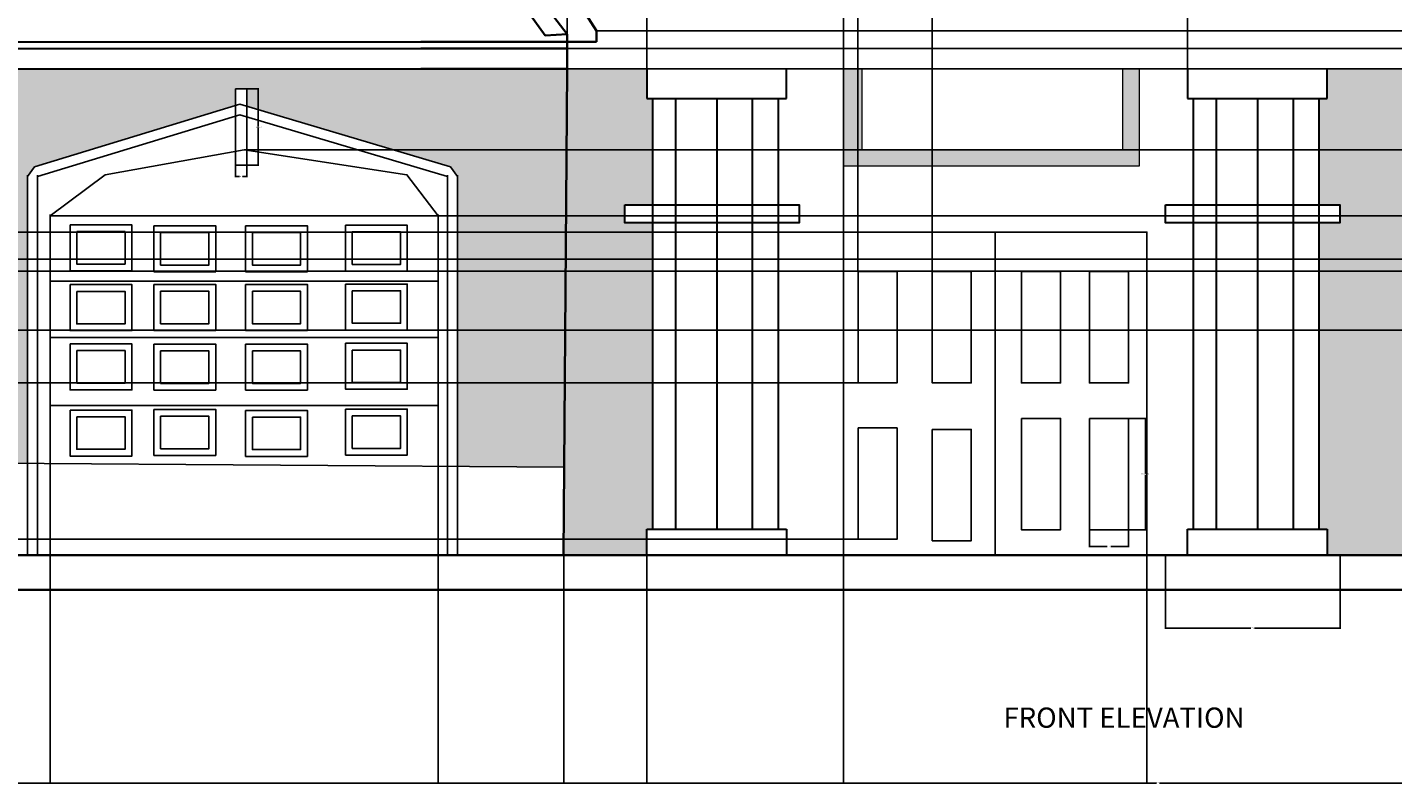
# Model space of a CAD drawing. Units: inches. Extents: x -46 to 1209, y 110 to 778.
# Tile 2 of 5: x 247 to 652, y 110 to 334. Entities that reach past the tile are written whole.
import ezdxf

# ---------------------------------------------------------------- set-up
doc = ezdxf.new("R2010")
doc.units = ezdxf.units.IN
doc.header["$MEASUREMENT"] = 0
for name, color, linetype, lineweight in [('A-ANNO-DIMS', 2, 'Continuous', 18), ('A-ANNO-TEXT', 7, 'Continuous', 25), ('A-COLS', 1, 'Continuous', 30), ('A-DOOR', 3, 'Continuous', 25), ('A-ELEV-BASE', 7, 'Continuous', 35), ('A-GLAZ', 4, 'Continuous', 20), ('A-GLAZ-PATT', 9, 'Continuous', 13), ('A-ROOF', 7, 'Continuous', 35), ('A-WALL', 7, 'Continuous', 35), ('A-WALL-PATT', 252, 'Continuous', 13), ('A-WALL-TRIM', 42, 'Continuous', 25)]:
    doc.layers.add(name, color=color, linetype=linetype, lineweight=lineweight)
doc.styles.get("Standard").update_dxf_attribs({"font": 'arial.ttf'})
doc.dimstyles.get("Standard").update_dxf_attribs({"dimtxt": 0.18, "dimasz": 0.18, "dimexe": 0.18, "dimexo": 0.0625, "dimgap": 0.09, "dimtad": 0, "dimtih": 1, "dimtoh": 1, "dimdec": 4, "dimzin": 0, "dimdsep": 46, "dimtxsty": 'Standard', "dimcen": 0.09, "dimadec": 0, "dimazin": 0, "dimtfac": 1, "dimtdec": 4, "dimtofl": 0, "dimtmove": 0, "dimatfit": 3, "dimfxl": 1, "dimtolj": 1, "dimtzin": 0, "dimarcsym": 0})

# ---------------------------------------------------------------- blocks, each defined once
blk = doc.blocks.new('COLUMN-ENTRY')
for p, q in [((6.6, 144.26), (6.6, 135.43)), ((48.01, 135.43), (48.01, 144.26)), ((6.6, 135.43), (48.01, 135.43)), ((8.21, 135.43), (8.21, 7.66)), ((15.08, 135.43), (15.08, 7.66)), ((27.3, 135.43), (27.3, 7.66)), ((37.85, 135.43), (37.85, 7.66)), ((45.52, 135.43), (45.52, 7.66)), ((6.6, 0), (6.6, 7.66)), ((6.6, 7.66), (48.01, 7.66)), ((48.01, 7.66), (48.01, 0))]:
    blk.add_line(p, q)
blk.add_lwpolyline([(0, 103.89), (51.79, 103.89), (51.79, 98.52), (0, 98.52)], close=True)
blk = doc.blocks.new('PANEL-GARAGE-RAISED')
for points in [[(0, 13.64), (18.32, 13.64), (18.32, 0), (0, 0)], [(2, 11.64), (16.32, 11.64), (16.32, 2), (2, 2)]]:
    blk.add_lwpolyline(points, close=True)
blk = doc.blocks.new('PANEL-ENTRY')
blk.add_lwpolyline([(0, 33.04), (11.61, 33.04), (11.61, 0), (0, 0)], close=True)
blk = doc.blocks.new('KEYSTONE-GARAGE')
blk.add_lwpolyline([(0, 22.61), (3.38, 22.61), (3.38, 0), (0, 0)], close=True)
blk = doc.blocks.new('*D14')
at = {"layer": 'A-ANNO-DIMS', "color": 0, "lineweight": -2, "transparency": 16777216}
for p, q in [((573.27, 218.29), (578.35, 218.29)), ((578.17, 218.11), (578.17, 201.95)), ((578.17, 185.43), (578.17, 201.59)), ((573.27, 185.25), (578.35, 185.25))]:
    blk.add_line(p, q, dxfattribs=at)
at = {"layer": 'A-ANNO-DIMS', "color": 0, "transparency": 16777216}
for points in [[(578.14, 218.11), (578.2, 218.11), (578.17, 218.29)], [(578.14, 185.43), (578.2, 185.43), (578.17, 185.25)]]:
    blk.add_solid(points, dxfattribs=at)
at = {"layer": 'Defpoints', "color": 0, "transparency": 16777216}
for p in [(573.21, 218.29), (578.17, 218.29), (573.21, 185.25)]:
    blk.add_point(p, dxfattribs=at)
at = {"layer": 'A-ANNO-DIMS', "color": 0, "transparency": 16777216, "insert": (578.17, 201.77), "char_height": 0.18, "attachment_point": 5}
blk.add_mtext('\\A1;ENTRY PANEL 33 TYP.', dxfattribs=at)
blk = doc.blocks.new('*D15')
at = {"layer": 'A-ANNO-DIMS', "color": 0, "lineweight": -2, "transparency": 16777216}
for p, q in [((561.6, 185.19), (561.6, 180.11)), ((573.21, 185.19), (573.21, 180.11)), ((561.78, 180.29), (566.89, 180.29)), ((573.03, 180.29), (567.93, 180.29))]:
    blk.add_line(p, q, dxfattribs=at)
at = {"layer": 'A-ANNO-DIMS', "color": 0, "transparency": 16777216}
for points in [[(561.78, 180.32), (561.78, 180.26), (561.6, 180.29)], [(573.03, 180.32), (573.03, 180.26), (573.21, 180.29)]]:
    blk.add_solid(points, dxfattribs=at)
at = {"layer": 'Defpoints', "color": 0, "transparency": 16777216}
for p in [(561.6, 185.25), (573.21, 185.25), (573.21, 180.29)]:
    blk.add_point(p, dxfattribs=at)
at = {"layer": 'A-ANNO-DIMS', "color": 0, "transparency": 16777216, "insert": (567.41, 180.29), "char_height": 0.18, "attachment_point": 5}
blk.add_mtext('\\A1;12 TYP.', dxfattribs=at)
blk = doc.blocks.new('*D22')
at = {"layer": 'A-ANNO-DIMS', "color": 0, "lineweight": -2, "transparency": 16777216}
for p, q in [((635.97, 321.99), (657.72, 321.99)), ((657.54, 321.81), (657.54, 250.04)), ((657.54, 177.91), (657.54, 249.68)), ((635.97, 177.73), (657.72, 177.73))]:
    blk.add_line(p, q, dxfattribs=at)
at = {"layer": 'A-ANNO-DIMS', "color": 0, "transparency": 16777216}
for points in [[(657.51, 321.81), (657.57, 321.81), (657.54, 321.99)], [(657.51, 177.91), (657.57, 177.91), (657.54, 177.73)]]:
    blk.add_solid(points, dxfattribs=at)
at = {"layer": 'Defpoints', "color": 0, "transparency": 16777216}
for p in [(635.91, 321.99), (657.54, 321.99), (635.91, 177.73)]:
    blk.add_point(p, dxfattribs=at)
at = {"layer": 'A-ANNO-DIMS', "color": 0, "transparency": 16777216, "insert": (657.54, 249.86), "char_height": 0.18, "attachment_point": 5}
blk.add_mtext('\\A1;ENTRY COLUMN 144 TYP.', dxfattribs=at)
blk = doc.blocks.new('*D23')
at = {"layer": 'A-ANNO-DIMS', "color": 0, "lineweight": -2, "transparency": 16777216}
for p, q in [((584.12, 177.67), (584.12, 155.91)), ((635.91, 177.67), (635.91, 155.91)), ((584.3, 156.09), (609.48, 156.09)), ((635.73, 156.09), (610.54, 156.09))]:
    blk.add_line(p, q, dxfattribs=at)
at = {"layer": 'A-ANNO-DIMS', "color": 0, "transparency": 16777216}
for points in [[(584.3, 156.12), (584.3, 156.06), (584.12, 156.09)], [(635.73, 156.12), (635.73, 156.06), (635.91, 156.09)]]:
    blk.add_solid(points, dxfattribs=at)
at = {"layer": 'Defpoints', "color": 0, "transparency": 16777216}
for p in [(584.12, 177.73), (635.91, 177.73), (635.91, 156.09)]:
    blk.add_point(p, dxfattribs=at)
at = {"layer": 'A-ANNO-DIMS', "color": 0, "transparency": 16777216, "insert": (610.01, 156.09), "char_height": 0.18, "attachment_point": 5}
blk.add_mtext('\\A1;52 TYP.', dxfattribs=at)
blk = doc.blocks.new('*D24')
at = {"layer": 'A-ANNO-DIMS', "color": 0, "lineweight": -2, "transparency": 16777216}
for p, q in [((311.69, 316.01), (315.2, 316.01)), ((315.02, 315.83), (315.02, 304.89)), ((315.02, 293.58), (315.02, 304.52)), ((311.69, 293.4), (315.2, 293.4))]:
    blk.add_line(p, q, dxfattribs=at)
at = {"layer": 'A-ANNO-DIMS', "color": 0, "transparency": 16777216}
for points in [[(314.99, 315.83), (315.05, 315.83), (315.02, 316.01)], [(314.99, 293.58), (315.05, 293.58), (315.02, 293.4)]]:
    blk.add_solid(points, dxfattribs=at)
at = {"layer": 'Defpoints', "color": 0, "transparency": 16777216}
for p in [(311.63, 316.01), (315.02, 316.01), (311.63, 293.4)]:
    blk.add_point(p, dxfattribs=at)
at = {"layer": 'A-ANNO-DIMS', "color": 0, "transparency": 16777216, "insert": (315.02, 304.71), "char_height": 0.18, "attachment_point": 5}
blk.add_mtext('\\A1;KEYSTONE 23 TYP.', dxfattribs=at)
blk = doc.blocks.new('*D25')
at = {"layer": 'A-ANNO-DIMS', "color": 0, "lineweight": -2, "transparency": 16777216}
for p, q in [((308.25, 293.34), (308.25, 289.83)), ((311.63, 293.34), (311.63, 289.83)), ((308.43, 290.01), (309.48, 290.01)), ((311.45, 290.01), (310.4, 290.01))]:
    blk.add_line(p, q, dxfattribs=at)
at = {"layer": 'A-ANNO-DIMS', "color": 0, "transparency": 16777216}
for points in [[(308.43, 290.04), (308.43, 289.98), (308.25, 290.01)], [(311.45, 290.04), (311.45, 289.98), (311.63, 290.01)]]:
    blk.add_solid(points, dxfattribs=at)
at = {"layer": 'Defpoints', "color": 0, "transparency": 16777216}
for p in [(308.25, 293.4), (311.63, 293.4), (311.63, 290.01)]:
    blk.add_point(p, dxfattribs=at)
at = {"layer": 'A-ANNO-DIMS', "color": 0, "transparency": 16777216, "insert": (309.94, 290.01), "char_height": 0.18, "attachment_point": 5}
blk.add_mtext('\\A1;3 TYP.', dxfattribs=at)
blk = doc.blocks.new('*D28')
at = {"layer": 'A-ANNO-DIMS', "color": 0, "lineweight": -2, "transparency": 16777216}
for p, q in [((11.98, 329.67), (11.98, 109.96)), ((1151.8, 167.37), (1151.8, 109.96)), ((12.16, 110.14), (581.44, 110.14)), ((1151.62, 110.14), (582.35, 110.14))]:
    blk.add_line(p, q, dxfattribs=at)
at = {"layer": 'A-ANNO-DIMS', "color": 0, "transparency": 16777216}
for points in [[(12.16, 110.17), (12.16, 110.11), (11.98, 110.14)], [(1151.62, 110.17), (1151.62, 110.11), (1151.8, 110.14)]]:
    blk.add_solid(points, dxfattribs=at)
at = {"layer": 'Defpoints', "color": 0, "transparency": 16777216}
for p in [(11.98, 329.73), (1151.8, 167.44), (1151.8, 110.14)]:
    blk.add_point(p, dxfattribs=at)
at = {"layer": 'A-ANNO-DIMS', "color": 0, "transparency": 16777216, "insert": (581.89, 110.14), "char_height": 0.18, "attachment_point": 5}
blk.add_mtext('\\A1;1139.8', dxfattribs=at)
blk = doc.blocks.new('*D29')
at = {"layer": 'A-ANNO-DIMS', "color": 0, "lineweight": -2, "transparency": 16777216}
for p, q in [((456.52, 720.07), (-45.5, 720.07)), ((-45.32, 719.89), (-45.32, 443.93)), ((-45.32, 167.62), (-45.32, 443.57)), ((15.16, 167.44), (-45.5, 167.44))]:
    blk.add_line(p, q, dxfattribs=at)
at = {"layer": 'A-ANNO-DIMS', "color": 0, "transparency": 16777216}
for points in [[(-45.35, 719.89), (-45.29, 719.89), (-45.32, 720.07)], [(-45.35, 167.62), (-45.29, 167.62), (-45.32, 167.44)]]:
    blk.add_solid(points, dxfattribs=at)
at = {"layer": 'Defpoints', "color": 0, "transparency": 16777216}
for p in [(-45.32, 720.07), (456.58, 720.07), (15.23, 167.44)]:
    blk.add_point(p, dxfattribs=at)
at = {"layer": 'A-ANNO-DIMS', "color": 0, "transparency": 16777216, "insert": (-45.32, 443.75), "char_height": 0.18, "attachment_point": 5}
blk.add_mtext('\\A1;552.6', dxfattribs=at)
blk = doc.blocks.new('*D32')
at = {"layer": 'A-ANNO-DIMS', "color": 0, "lineweight": -2, "transparency": 16777216}
for p, q in [((209.64, 177.67), (209.64, 109.96)), ((253.32, 177.67), (253.32, 109.96)), ((209.82, 110.14), (231.08, 110.14)), ((253.14, 110.14), (231.88, 110.14))]:
    blk.add_line(p, q, dxfattribs=at)
at = {"layer": 'A-ANNO-DIMS', "color": 0, "transparency": 16777216}
for points in [[(209.82, 110.17), (209.82, 110.11), (209.64, 110.14)], [(253.14, 110.17), (253.14, 110.11), (253.32, 110.14)]]:
    blk.add_solid(points, dxfattribs=at)
at = {"layer": 'Defpoints', "color": 0, "transparency": 16777216}
for p in [(209.64, 177.73), (253.32, 177.73), (253.32, 110.14)]:
    blk.add_point(p, dxfattribs=at)
at = {"layer": 'A-ANNO-DIMS', "color": 0, "transparency": 16777216, "insert": (231.48, 110.14), "char_height": 0.18, "attachment_point": 5}
blk.add_mtext('\\A1;43.68', dxfattribs=at)
blk = doc.blocks.new('*D33')
at = {"layer": 'A-ANNO-DIMS', "color": 0, "lineweight": -2, "transparency": 16777216}
for p, q in [((253.32, 177.67), (253.32, 109.96)), ((368.44, 177.67), (368.44, 109.96)), ((253.5, 110.14), (310.43, 110.14)), ((368.26, 110.14), (311.34, 110.14))]:
    blk.add_line(p, q, dxfattribs=at)
at = {"layer": 'A-ANNO-DIMS', "color": 0, "transparency": 16777216}
for points in [[(253.5, 110.17), (253.5, 110.11), (253.32, 110.14)], [(368.26, 110.17), (368.26, 110.11), (368.44, 110.14)]]:
    blk.add_solid(points, dxfattribs=at)
at = {"layer": 'Defpoints', "color": 0, "transparency": 16777216}
for p in [(253.32, 177.73), (368.44, 177.73), (368.44, 110.14)]:
    blk.add_point(p, dxfattribs=at)
at = {"layer": 'A-ANNO-DIMS', "color": 0, "transparency": 16777216, "insert": (310.88, 110.14), "char_height": 0.18, "attachment_point": 5}
blk.add_mtext('\\A1;115.12', dxfattribs=at)
blk = doc.blocks.new('*D34')
at = {"layer": 'A-ANNO-DIMS', "color": 0, "lineweight": -2, "transparency": 16777216}
for p, q in [((368.44, 177.67), (368.44, 109.96)), ((405.63, 177.67), (405.63, 109.96)), ((368.62, 110.14), (386.64, 110.14)), ((405.45, 110.14), (387.43, 110.14))]:
    blk.add_line(p, q, dxfattribs=at)
at = {"layer": 'A-ANNO-DIMS', "color": 0, "transparency": 16777216}
for points in [[(368.62, 110.17), (368.62, 110.11), (368.44, 110.14)], [(405.45, 110.17), (405.45, 110.11), (405.63, 110.14)]]:
    blk.add_solid(points, dxfattribs=at)
at = {"layer": 'Defpoints', "color": 0, "transparency": 16777216}
for p in [(368.44, 177.73), (405.63, 177.73), (405.63, 110.14)]:
    blk.add_point(p, dxfattribs=at)
at = {"layer": 'A-ANNO-DIMS', "color": 0, "transparency": 16777216, "insert": (387.03, 110.14), "char_height": 0.18, "attachment_point": 5}
blk.add_mtext('\\A1;37.18', dxfattribs=at)
blk = doc.blocks.new('*D35')
at = {"layer": 'A-ANNO-DIMS', "color": 0, "lineweight": -2, "transparency": 16777216}
for p, q in [((368.5, 278.33), (1209.28, 278.33)), ((1209.1, 278.15), (1209.1, 228.21)), ((1209.1, 177.91), (1209.1, 227.85)), ((368.5, 177.73), (1209.28, 177.73))]:
    blk.add_line(p, q, dxfattribs=at)
at = {"layer": 'A-ANNO-DIMS', "color": 0, "transparency": 16777216}
for points in [[(1209.07, 278.15), (1209.13, 278.15), (1209.1, 278.33)], [(1209.07, 177.91), (1209.13, 177.91), (1209.1, 177.73)]]:
    blk.add_solid(points, dxfattribs=at)
at = {"layer": 'Defpoints', "color": 0, "transparency": 16777216}
for p in [(368.44, 278.33), (1209.1, 278.33), (368.44, 177.73)]:
    blk.add_point(p, dxfattribs=at)
at = {"layer": 'A-ANNO-DIMS', "color": 0, "transparency": 16777216, "insert": (1209.1, 228.03), "char_height": 0.18, "attachment_point": 5}
blk.add_mtext('\\A1;100.6', dxfattribs=at)
blk = doc.blocks.new('*D36')
at = {"layer": 'A-ANNO-DIMS', "color": 0, "lineweight": -2, "transparency": 16777216}
for p, q in [((310.94, 297.96), (1209.28, 297.96)), ((1209.1, 297.78), (1209.1, 288.33)), ((1209.1, 278.51), (1209.1, 287.96)), ((368.5, 278.33), (1209.28, 278.33))]:
    blk.add_line(p, q, dxfattribs=at)
at = {"layer": 'A-ANNO-DIMS', "color": 0, "transparency": 16777216}
for points in [[(1209.07, 297.78), (1209.13, 297.78), (1209.1, 297.96)], [(1209.07, 278.51), (1209.13, 278.51), (1209.1, 278.33)]]:
    blk.add_solid(points, dxfattribs=at)
at = {"layer": 'Defpoints', "color": 0, "transparency": 16777216}
for p in [(310.88, 297.96), (1209.1, 297.96), (368.44, 278.33)]:
    blk.add_point(p, dxfattribs=at)
at = {"layer": 'A-ANNO-DIMS', "color": 0, "transparency": 16777216, "insert": (1209.1, 288.14), "char_height": 0.18, "attachment_point": 5}
blk.add_mtext('\\A1;19.63', dxfattribs=at)
blk = doc.blocks.new('*D41')
at = {"layer": 'A-ANNO-DIMS', "color": 0, "lineweight": -2, "transparency": 16777216}
for p, q in [((198.93, 261.94), (1209.28, 261.94)), ((1209.1, 261.76), (1209.1, 253.4)), ((1209.1, 244.67), (1209.1, 253.04)), ((198.93, 244.49), (1209.28, 244.49))]:
    blk.add_line(p, q, dxfattribs=at)
at = {"layer": 'A-ANNO-DIMS', "color": 0, "transparency": 16777216}
for points in [[(1209.07, 261.76), (1209.13, 261.76), (1209.1, 261.94)], [(1209.07, 244.67), (1209.13, 244.67), (1209.1, 244.49)]]:
    blk.add_solid(points, dxfattribs=at)
at = {"layer": 'Defpoints', "color": 0, "transparency": 16777216}
for p in [(198.86, 261.94), (1209.1, 261.94), (198.86, 244.49)]:
    blk.add_point(p, dxfattribs=at)
at = {"layer": 'A-ANNO-DIMS', "color": 0, "transparency": 16777216, "insert": (1209.1, 253.22), "char_height": 0.18, "attachment_point": 5}
blk.add_mtext('\\A1;17.446', dxfattribs=at)
blk = doc.blocks.new('*D44')
at = {"layer": 'A-ANNO-DIMS', "color": 0, "lineweight": -2, "transparency": 16777216}
for p, q in [((18.95, 265.48), (1209.28, 265.48)), ((1209.1, 265.3), (1209.1, 221.79)), ((1209.1, 177.91), (1209.1, 221.42)), ((15.29, 177.73), (1209.28, 177.73))]:
    blk.add_line(p, q, dxfattribs=at)
at = {"layer": 'A-ANNO-DIMS', "color": 0, "transparency": 16777216}
for points in [[(1209.07, 265.3), (1209.13, 265.3), (1209.1, 265.48)], [(1209.07, 177.91), (1209.13, 177.91), (1209.1, 177.73)]]:
    blk.add_solid(points, dxfattribs=at)
at = {"layer": 'Defpoints', "color": 0, "transparency": 16777216}
for p in [(18.89, 265.48), (1209.1, 265.48), (15.23, 177.73)]:
    blk.add_point(p, dxfattribs=at)
at = {"layer": 'A-ANNO-DIMS', "color": 0, "transparency": 16777216, "insert": (1209.1, 221.6), "char_height": 0.18, "attachment_point": 5}
blk.add_mtext('\\A1;87.74', dxfattribs=at)
blk = doc.blocks.new('*D46')
at = {"layer": 'A-ANNO-DIMS', "color": 0, "lineweight": -2, "transparency": 16777216}
for p, q in [((406.65, 322.05), (406.65, 777.55)), ((406.83, 777.37), (447.43, 777.37)), ((488.47, 777.37), (447.87, 777.37)), ((488.65, 273.58), (488.65, 777.55))]:
    blk.add_line(p, q, dxfattribs=at)
at = {"layer": 'A-ANNO-DIMS', "color": 0, "transparency": 16777216}
for points in [[(406.83, 777.4), (406.83, 777.34), (406.65, 777.37)], [(488.47, 777.4), (488.47, 777.34), (488.65, 777.37)]]:
    blk.add_solid(points, dxfattribs=at)
at = {"layer": 'Defpoints', "color": 0, "transparency": 16777216}
for p in [(488.65, 777.37), (406.65, 321.99), (488.65, 273.51)]:
    blk.add_point(p, dxfattribs=at)
at = {"layer": 'A-ANNO-DIMS', "color": 0, "transparency": 16777216, "insert": (447.65, 777.37), "char_height": 0.18, "attachment_point": 5}
blk.add_mtext('\\A1;82', dxfattribs=at)
blk = doc.blocks.new('*D47')
at = {"layer": 'A-ANNO-DIMS', "color": 0, "lineweight": -2, "transparency": 16777216}
for p, q in [((430.32, 177.67), (430.32, 109.96)), ((488.65, 177.67), (488.65, 109.96)), ((430.5, 110.14), (459.09, 110.14)), ((488.47, 110.14), (459.88, 110.14))]:
    blk.add_line(p, q, dxfattribs=at)
at = {"layer": 'A-ANNO-DIMS', "color": 0, "transparency": 16777216}
for points in [[(430.5, 110.17), (430.5, 110.11), (430.32, 110.14)], [(488.47, 110.17), (488.47, 110.11), (488.65, 110.14)]]:
    blk.add_solid(points, dxfattribs=at)
at = {"layer": 'Defpoints', "color": 0, "transparency": 16777216}
for p in [(430.32, 177.73), (488.65, 177.73), (488.65, 110.14)]:
    blk.add_point(p, dxfattribs=at)
at = {"layer": 'A-ANNO-DIMS', "color": 0, "transparency": 16777216, "insert": (459.49, 110.14), "char_height": 0.18, "attachment_point": 5}
blk.add_mtext('\\A1;58.33', dxfattribs=at)
blk = doc.blocks.new('*D48')
at = {"layer": 'A-ANNO-DIMS', "color": 0, "lineweight": -2, "transparency": 16777216}
for p, q in [((488.65, 177.67), (488.65, 109.96)), ((578.65, 177.67), (578.65, 109.96)), ((488.83, 110.14), (533.43, 110.14)), ((578.47, 110.14), (533.87, 110.14))]:
    blk.add_line(p, q, dxfattribs=at)
at = {"layer": 'A-ANNO-DIMS', "color": 0, "transparency": 16777216}
for points in [[(488.83, 110.17), (488.83, 110.11), (488.65, 110.14)], [(578.47, 110.17), (578.47, 110.11), (578.65, 110.14)]]:
    blk.add_solid(points, dxfattribs=at)
at = {"layer": 'Defpoints', "color": 0, "transparency": 16777216}
for p in [(488.65, 177.73), (578.65, 177.73), (578.65, 110.14)]:
    blk.add_point(p, dxfattribs=at)
at = {"layer": 'A-ANNO-DIMS', "color": 0, "transparency": 16777216, "insert": (533.65, 110.14), "char_height": 0.18, "attachment_point": 5}
blk.add_mtext('\\A1;90', dxfattribs=at)
blk = doc.blocks.new('*D49')
at = {"layer": 'A-ANNO-DIMS', "color": 0, "lineweight": -2, "transparency": 16777216}
for p, q in [((488.59, 273.51), (-45.5, 273.51)), ((-45.32, 273.33), (-45.32, 225.8)), ((-45.32, 177.91), (-45.32, 225.44)), ((488.59, 177.73), (-45.5, 177.73))]:
    blk.add_line(p, q, dxfattribs=at)
at = {"layer": 'A-ANNO-DIMS', "color": 0, "transparency": 16777216}
for points in [[(-45.35, 273.33), (-45.29, 273.33), (-45.32, 273.51)], [(-45.35, 177.91), (-45.29, 177.91), (-45.32, 177.73)]]:
    blk.add_solid(points, dxfattribs=at)
at = {"layer": 'Defpoints', "color": 0, "transparency": 16777216}
for p in [(-45.32, 273.51), (488.65, 273.51), (488.65, 177.73)]:
    blk.add_point(p, dxfattribs=at)
at = {"layer": 'A-ANNO-DIMS', "color": 0, "transparency": 16777216, "insert": (-45.32, 225.62), "char_height": 0.18, "attachment_point": 5}
blk.add_mtext('\\A1;95.78', dxfattribs=at)
blk = doc.blocks.new('*D50')
at = {"layer": 'A-ANNO-DIMS', "color": 0, "lineweight": -2, "transparency": 16777216}
for p, q in [((430.32, 322.05), (430.32, 777.55)), ((430.5, 777.37), (510.13, 777.37)), ((590.53, 777.37), (510.9, 777.37)), ((590.71, 322.05), (590.71, 777.55))]:
    blk.add_line(p, q, dxfattribs=at)
at = {"layer": 'A-ANNO-DIMS', "color": 0, "transparency": 16777216}
for points in [[(430.5, 777.4), (430.5, 777.34), (430.32, 777.37)], [(590.53, 777.4), (590.53, 777.34), (590.71, 777.37)]]:
    blk.add_solid(points, dxfattribs=at)
at = {"layer": 'Defpoints', "color": 0, "transparency": 16777216}
for p in [(590.71, 777.37), (430.32, 321.99), (590.71, 321.99)]:
    blk.add_point(p, dxfattribs=at)
at = {"layer": 'A-ANNO-DIMS', "color": 0, "transparency": 16777216, "insert": (510.52, 777.37), "char_height": 0.18, "attachment_point": 5}
blk.add_mtext('\\A1;160.4', dxfattribs=at)
blk = doc.blocks.new('*D51')
at = {"layer": 'A-ANNO-DIMS', "color": 0, "lineweight": -2, "transparency": 16777216}
for p, q in [((492.93, 261.94), (492.93, 777.55)), ((493.11, 777.37), (503.47, 777.37)), ((514.76, 777.37), (504.4, 777.37)), ((514.94, 261.94), (514.94, 777.55))]:
    blk.add_line(p, q, dxfattribs=at)
at = {"layer": 'A-ANNO-DIMS', "color": 0, "transparency": 16777216}
for points in [[(493.11, 777.4), (493.11, 777.34), (492.93, 777.37)], [(514.76, 777.4), (514.76, 777.34), (514.94, 777.37)]]:
    blk.add_solid(points, dxfattribs=at)
at = {"layer": 'Defpoints', "color": 0, "transparency": 16777216}
for p in [(514.94, 777.37), (492.93, 261.87), (514.94, 261.87)]:
    blk.add_point(p, dxfattribs=at)
at = {"layer": 'A-ANNO-DIMS', "color": 0, "transparency": 16777216, "insert": (503.94, 777.37), "char_height": 0.18, "attachment_point": 5}
blk.add_mtext('\\A1;22.003', dxfattribs=at)
blk = doc.blocks.new('*D52')
at = {"layer": 'A-ANNO-DIMS', "color": 0, "lineweight": -2, "transparency": 16777216}
for p, q in [((492.87, 228.83), (-45.5, 228.83)), ((-45.32, 228.65), (-45.32, 205.81)), ((-45.32, 182.61), (-45.32, 205.45)), ((492.87, 182.43), (-45.5, 182.43))]:
    blk.add_line(p, q, dxfattribs=at)
at = {"layer": 'A-ANNO-DIMS', "color": 0, "transparency": 16777216}
for points in [[(-45.35, 228.65), (-45.29, 228.65), (-45.32, 228.83)], [(-45.35, 182.61), (-45.29, 182.61), (-45.32, 182.43)]]:
    blk.add_solid(points, dxfattribs=at)
at = {"layer": 'Defpoints', "color": 0, "transparency": 16777216}
for p in [(-45.32, 228.83), (492.93, 228.83), (492.93, 182.43)]:
    blk.add_point(p, dxfattribs=at)
at = {"layer": 'A-ANNO-DIMS', "color": 0, "transparency": 16777216, "insert": (-45.32, 205.63), "char_height": 0.18, "attachment_point": 5}
blk.add_mtext('\\A1;46.4', dxfattribs=at)

msp = doc.modelspace()

# ---------------------------------------------------------------- hatches: boundary and pattern name
at = {"layer": 'A-GLAZ-PATT'}
h = msp.add_hatch(color=256, dxfattribs=at)
h.dxf.hatch_style = 1
h.paths.add_polyline_path([(576.3018, 321.9907), (571.484, 321.9907), (571.484, 297.8828), (494.057, 297.8828), (494.057, 321.9907), (488.6503, 321.9907), (488.6503, 293.0961), (576.3018, 293.0961)])
at = {"layer": 'A-WALL-PATT'}
h = msp.add_hatch(dxfattribs=at)
h.set_pattern_fill('AR-CONC', color=256, scale=3)
h.paths.add_polyline_path([(387.8322, 595.7911), (179.1007, 595.7911), (179.1007, 451.7911), (179.1007, 439.7911), (220.892, 454.7186), (313.6366, 436.1845), (387.8322, 376.346)])
h.paths.add_polyline_path([(276.7646, 548.5945), (292.8821, 548.5945), (292.8821, 553.0308), (295.9402, 553.0308), (295.9402, 548.5945), (313.3682, 548.5945), (313.3682, 512.6263), (276.7646, 512.6263)], flags=16)
h.paths.add_polyline_path([(278.6627, 545.0233), (312.1316, 545.0233), (312.1316, 514.6792), (278.6627, 514.6792)], flags=0)
h.paths.add_polyline_path([(326.2691, 548.5945), (341.5129, 548.5945), (341.5129, 553.0308), (344.571, 553.0308), (344.571, 548.5945), (362.8728, 548.5945), (362.8728, 512.6263), (326.2691, 512.6263)], flags=16)
h.paths.add_polyline_path([(328.1673, 545.0233), (361.6362, 545.0233), (361.6362, 514.6792), (328.1673, 514.6792)], flags=0)
h.paths.add_polyline_path([(651.5361, 595.7911), (415.401, 595.7911), (387.8322, 595.7911), (387.8322, 376.346), (409.6414, 342.2631), (651.5361, 342.2631)])
h.paths.add_polyline_path([(470.5081, 534.2042), (467.0793, 534.2042), (467.0793, 554.4029), (483.2058, 554.4029), (483.2058, 549.2024), (518.0634, 549.2024), (518.0634, 557.4852), (520.3257, 557.4852), (520.3257, 564.6435), (523.2165, 564.6435), (523.2165, 557.4852), (525.4788, 557.4852), (525.4788, 549.2024), (567.4184, 549.2024), (567.4184, 554.4029), (579.1691, 554.4029), (579.1691, 534.2042), (575.9249, 534.2042), (575.9249, 428.1662), (580.259, 428.1662), (580.259, 412.8567), (567.4184, 412.8567), (567.4184, 417.1318), (483.8186, 417.1318), (483.8186, 413.5449), (465.7589, 413.5449), (465.7589, 426.3336), (470.5081, 426.3336)], flags=16)
h.paths.add_polyline_path([(483.2375, 532.926), (568.2834, 532.926), (568.2834, 425.5857), (483.2375, 425.5857)], flags=0)
h.paths.add_polyline_path([(431.7717, 578.8147), (431.7717, 585.9699), (440.9467, 585.9699), (440.9467, 578.8147)], flags=16)
h.paths.add_polyline_path([(423.2681, 578.8147), (414.0931, 578.8147), (414.0931, 585.9699), (423.2681, 585.9699)], flags=16)
h.paths.add_polyline_path([(447.8839, 578.8147), (447.8839, 585.9699), (457.0589, 585.9699), (457.0589, 578.8147)], flags=16)
h.paths.add_polyline_path([(406.5964, 578.8147), (397.4214, 578.8147), (397.4214, 585.9699), (406.5964, 585.9699)], flags=16)
h.paths.add_polyline_path([(466.0101, 578.8147), (466.0101, 585.9699), (475.1851, 585.9699), (475.1851, 578.8147)], flags=16)
h.paths.add_polyline_path([(483.6888, 578.8147), (483.6888, 585.9699), (492.8638, 585.9699), (492.8638, 578.8147)], flags=16)
h.paths.add_polyline_path([(504.0528, 578.8147), (504.0528, 585.9699), (513.2278, 585.9699), (513.2278, 578.8147)], flags=16)
h.paths.add_polyline_path([(523.0742, 578.8147), (523.0742, 585.9699), (532.2492, 585.9699), (532.2492, 578.8147)], flags=16)
h.paths.add_polyline_path([(542.3193, 578.8147), (542.3193, 585.9699), (551.4943, 585.9699), (551.4943, 578.8147)], flags=16)
h.paths.add_polyline_path([(559.998, 578.8147), (559.998, 585.9699), (569.1729, 585.9699), (569.1729, 578.8147)], flags=16)
h.paths.add_polyline_path([(580.1382, 578.8147), (580.1382, 585.9699), (589.3132, 585.9699), (589.3132, 578.8147)], flags=16)
h.paths.add_polyline_path([(598.3313, 578.8147), (598.3313, 585.9699), (607.5063, 585.9699), (607.5063, 578.8147)], flags=16)
h.paths.add_polyline_path([(618.2477, 578.8147), (618.2477, 585.9699), (627.4227, 585.9699), (627.4227, 578.8147)], flags=16)
h.paths.add_polyline_path([(636.8215, 578.8147), (636.8215, 585.9699), (645.9965, 585.9699), (645.9965, 578.8147)], flags=16)
h.paths.add_polyline_path([(1151.8016, 595.7911), (651.5361, 595.7911), (651.5361, 342.2631), (939.9139, 342.2631), (1151.8016, 342.2631)])
h.paths.add_polyline_path([(683.9631, 455.0835), (683.9631, 537.4823), (720.8864, 537.4823), (720.8864, 547.6453), (727.8922, 547.6453), (727.8922, 537.4823), (767.8177, 537.4823), (767.8177, 455.0835)], flags=16)
h.paths.add_polyline_path([(688.3115, 459.7865), (688.3115, 529.3012), (764.9847, 529.3012), (764.9847, 459.7865)], flags=0)
h.paths.add_polyline_path([(840.5045, 455.0835), (840.5045, 537.4823), (877.4279, 537.4823), (877.4279, 547.6453), (884.4336, 547.6453), (884.4336, 537.4823), (924.3592, 537.4823), (924.3592, 455.0835)], flags=16)
h.paths.add_polyline_path([(844.853, 459.7865), (844.853, 529.3012), (921.5262, 529.3012), (921.5262, 459.7865)], flags=0)
h.paths.add_polyline_path([(994.2223, 455.0835), (994.2223, 537.4823), (1031.1457, 537.4823), (1031.1457, 547.6453), (1038.1514, 547.6453), (1038.1514, 537.4823), (1078.077, 537.4823), (1078.077, 455.0835)], flags=16)
h.paths.add_polyline_path([(998.5708, 459.7865), (998.5708, 529.3012), (1075.244, 529.3012), (1075.244, 459.7865)], flags=0)
h.paths.add_polyline_path([(1151.8016, 321.9907), (941.4829, 321.9907), (632.1261, 321.9907), (632.1261, 313.1625), (629.6322, 313.1625), (629.6322, 281.6236), (635.9059, 281.6236), (635.9059, 276.2471), (629.6322, 276.2471), (629.6322, 185.3878), (632.1261, 185.3878), (632.1261, 177.7316), (1151.8016, 177.7316)])
h.paths.add_polyline_path([(704.3294, 282.1806), (702.3037, 282.1806), (702.3037, 292.8947), (707.3294, 292.8947), (707.3294, 290.4743), (740.8704, 290.4743), (740.8704, 292.7856), (747.2108, 292.7856), (747.2108, 281.5404), (744.5274, 281.5404), (744.5274, 216.7007), (746.4513, 216.7007), (746.4513, 208.2103), (741.5274, 208.2103), (741.5274, 210.4615), (707.3294, 210.4615), (707.3294, 208.0997), (702.1613, 208.0997), (702.1613, 216.7007), (704.3294, 216.7007)], flags=16)
h.paths.add_polyline_path([(707.3294, 287.4743), (741.5274, 287.4743), (741.5274, 213.4615), (707.3294, 213.4615)], flags=0)
h.paths.add_polyline_path([(859.0635, 282.1806), (859.0635, 292.8947), (864.0892, 292.8947), (864.0892, 290.4743), (897.6301, 290.4743), (897.6301, 292.7856), (903.9705, 292.7856), (903.9705, 281.5404), (901.2871, 281.5404), (901.2871, 216.7007), (903.2111, 216.7007), (903.2111, 208.2103), (898.2871, 208.2103), (898.2871, 210.4615), (864.0892, 210.4615), (864.0892, 208.0997), (858.9211, 208.0997), (858.9211, 216.7007), (861.0892, 216.7007), (861.0892, 282.1806)], flags=16)
h.paths.add_polyline_path([(864.0892, 287.4743), (898.2871, 287.4743), (898.2871, 213.4615), (864.0892, 213.4615)], flags=0)
h.paths.add_polyline_path([(1013.4529, 282.1806), (1013.4529, 292.8947), (1018.4786, 292.8947), (1018.4786, 290.4743), (1052.0195, 290.4743), (1052.0195, 292.7856), (1058.3599, 292.7856), (1058.3599, 281.5404), (1055.6765, 281.5404), (1055.6765, 216.7007), (1057.6005, 216.7007), (1057.6005, 208.2103), (1052.6765, 208.2103), (1052.6765, 210.4615), (1018.4786, 210.4615), (1018.4786, 208.0997), (1013.3105, 208.0997), (1013.3105, 216.7007), (1015.4786, 216.7007), (1015.4786, 282.1806)], flags=16)
h.paths.add_polyline_path([(1018.4786, 287.4743), (1052.6765, 287.4743), (1052.6765, 213.4615), (1018.4786, 213.4615)], flags=0)
h.paths.add_polyline_path([(431.9367, 276.2471), (423.7231, 276.2471), (423.7231, 281.6236), (431.9367, 281.6236), (431.9367, 313.1625), (430.3199, 313.1625), (430.3199, 321.9907), (406.6462, 321.9907), (406.6462, 321.7316), (405.6256, 177.7316), (430.3199, 177.7316), (430.3199, 185.3878), (431.9367, 185.3878)])
h.paths.add_polyline_path([(406.6462, 321.7316), (406.6462, 321.9907), (363.2774, 321.9907), (58.5947, 321.7316), (57.7764, 206.2827), (87.7834, 206.0701), (87.7834, 290.4607), (89.9075, 293.33), (149.9611, 311.663), (149.9611, 316.8909), (153.3383, 316.8909), (153.3383, 311.1504), (213.2336, 293.3362), (215.3783, 290.4607), (215.3783, 205.1657), (246.588, 204.9445), (246.588, 290.0127), (248.7121, 292.882), (308.2509, 311.0579), (308.2509, 316.0122), (311.6281, 316.0122), (311.6281, 310.8556), (372.0381, 292.8882), (374.1829, 290.0127), (374.1829, 204.0402), (405.8105, 203.8161)])
h.paths.add_polyline_path([(333, 359.5), (292.5, 377), (250.5, 387.5), (199, 387.5), (155, 377.5), (123.5, 364), (101.4287, 342.2631), (363.2774, 342.2631)])
h.paths.add_polyline_path([(579.9721, 681.6773), (549.8011, 690.7996), (524.9646, 691.17), (482.8908, 691.7975), (447.0968, 679.2482), (416.3264, 659.1694), (597.1807, 659.1694)])

# ---------------------------------------------------------------- linework, layer by layer
at = {"layer": 'A-DOOR'}
for p, q in [((246.588, 290.0127), (248.7121, 292.882)), ((372.0381, 292.8882), (374.1829, 290.0127)), ((246.588, 177.7316), (246.588, 290.4607)), ((249.588, 177.7316), (249.588, 290.4607)), ((371.1829, 177.7316), (371.1829, 290.4607)), ((374.1829, 177.7316), (374.1829, 290.4607)), ((253.3203, 177.7316), (253.3203, 278.7768)), ((253.3203, 278.3288), (368.4424, 278.3288)), ((368.4424, 278.7768), (368.4424, 177.7316)), ((533.6486, 273.5127), (533.6486, 177.7316)), ((253.3203, 259.002), (368.4424, 259.002)), ((253.3203, 242.3165), (368.4424, 242.3165)), ((253.3203, 222.0917), (368.4424, 222.0917))]:
    msp.add_line(p, q, dxfattribs=at)
for points in [[(248.7121, 292.882), (309.5817, 311.4642), (372.0381, 292.8882)], [(249.588, 290.0127), (309.593, 308.331), (371.1829, 290.0127)], [(253.3203, 278.3288), (269.5996, 290.5254), (310.8814, 297.9586)], [(368.4424, 278.3288), (359.1263, 290.5254), (310.8814, 297.9586)]]:
    msp.add_lwpolyline(points, dxfattribs=at)
msp.add_lwpolyline([(488.6503, 273.5127), (578.6468, 273.5127), (578.6468, 177.7316), (488.6503, 177.7316)], close=True, dxfattribs=at)
at = {"layer": 'A-ELEV-BASE'}
for p, q in [((15.2259, 177.7316), (1151.8016, 177.7316)), ((57.5741, 177.7316), (405.6256, 177.7316)), ((15.2259, 167.435), (1151.8016, 167.435))]:
    msp.add_line(p, q, dxfattribs=at)
at = {"layer": 'A-GLAZ'}
for p, q in [((494.057, 321.9907), (494.057, 297.8828)), ((571.484, 297.8828), (571.484, 321.9907)), ((494.057, 297.8828), (571.484, 297.8828))]:
    msp.add_line(p, q, dxfattribs=at)
msp.add_lwpolyline([(488.6503, 321.9907), (576.3018, 321.9907), (576.3018, 293.0961), (488.6503, 293.0961)], close=True, dxfattribs=at)
at = {"layer": 'A-ROOF'}
for p, q in [((406.7029, 332.2401), (400.1222, 331.7916)), ((406.7029, 329.9907), (406.7029, 332.2401)), ((415.401, 329.9907), (415.401, 333.2621)), ((363.2774, 329.9907), (58.6514, 329.7316)), ((363.2774, 329.9907), (406.7029, 329.9907)), ((402.1267, 329.9907), (405.0339, 329.9907)), ((406.7029, 329.9907), (406.6888, 327.9907)), ((406.7029, 329.9907), (415.401, 329.9907)), ((363.2632, 327.9907), (58.6372, 327.7316)), ((363.2774, 327.9907), (406.6888, 327.9907)), ((406.6888, 327.9907), (406.6462, 321.9907)), ((58.5947, 321.7316), (363.2774, 321.9907)), ((363.2774, 321.9907), (406.6462, 321.9907))]:
    msp.add_line(p, q, dxfattribs=at)
for points in [[(53.8945, 337.7316), (104.7154, 413.2214), (220.892, 454.7186), (313.6366, 436.1845), (387.8322, 376.346), (415.401, 333.2621)], [(56.9823, 332.8507), (113.0259, 401.4848), (221.8022, 437.979), (307.5529, 423.6986), (376.6298, 371.3374), (406.7029, 332.2401)], [(61.2975, 331.811), (115.3935, 398.06), (222.1289, 433.8695), (305.9227, 419.915), (373.7332, 368.5138), (400.1222, 331.7916)]]:
    msp.add_lwpolyline(points, dxfattribs=at)
at = {"layer": 'A-WALL'}
for p, q in [((406.6462, 321.7316), (405.6256, 177.7316)), ((406.6462, 321.9907), (406.6462, 321.7316))]:
    msp.add_line(p, q, dxfattribs=at)
at = {"layer": 'A-WALL-TRIM'}
for p, q in [((415.401, 333.2621), (933.8719, 333.2621)), ((406.6888, 327.9907), (918.2932, 327.9907)), ((406.6462, 321.9907), (941.4829, 321.9907)), ((57.7764, 206.2827), (405.8105, 203.8161))]:
    msp.add_line(p, q, dxfattribs=at)

# ---------------------------------------------------------------- block references
at = {"layer": 'A-COLS'}
for p in [(423.7231, 177.7316), (584.1152, 177.7316)]:
    msp.add_blockref('COLUMN-ENTRY', p, dxfattribs=at)
at = {"layer": 'A-DOOR'}
for name, p in [('KEYSTONE-GARAGE', (308.2509, 293.4032)), ('PANEL-GARAGE-RAISED', (259.2186, 262.0405)), ('PANEL-GARAGE-RAISED', (340.9284, 261.9412)), ('PANEL-GARAGE-RAISED', (284.0821, 261.7525)), ('PANEL-GARAGE-RAISED', (311.2777, 261.7525)), ('PANEL-ENTRY', (492.9346, 228.8283)), ('PANEL-ENTRY', (514.9372, 228.8283)), ('PANEL-ENTRY', (541.4001, 228.8283)), ('PANEL-ENTRY', (561.6018, 228.8283)), ('PANEL-GARAGE-RAISED', (259.2186, 244.3248)), ('PANEL-GARAGE-RAISED', (284.0821, 244.3697)), ('PANEL-GARAGE-RAISED', (311.2777, 244.3697)), ('PANEL-GARAGE-RAISED', (340.9284, 244.4949)), ('PANEL-GARAGE-RAISED', (259.2186, 226.7501)), ('PANEL-GARAGE-RAISED', (284.0821, 226.6796)), ('PANEL-GARAGE-RAISED', (311.2777, 226.6796)), ('PANEL-GARAGE-RAISED', (340.9284, 226.9259)), ('PANEL-GARAGE-RAISED', (259.2186, 207.1307)), ('PANEL-GARAGE-RAISED', (284.0821, 207.2931)), ('PANEL-GARAGE-RAISED', (311.2777, 207.0245)), ('PANEL-GARAGE-RAISED', (340.9284, 207.3838)), ('PANEL-ENTRY', (492.9346, 182.4306)), ('PANEL-ENTRY', (514.9372, 181.9942)), ('PANEL-ENTRY', (541.4001, 185.2499)), ('PANEL-ENTRY', (561.6018, 185.2499))]:
    msp.add_blockref(name, p, dxfattribs=at)

# ---------------------------------------------------------------- texts
at = {"layer": 'A-ANNO-TEXT', "insert": (536.0786, 132.5355), "char_height": 6, "attachment_point": 1}
msp.add_mtext_dynamic_manual_height_columns('FRONT ELEVATION', width=135.914595, gutter_width=1, heights=[0], dxfattribs=at)

# ---------------------------------------------------------------- dimensions: what is measured, and where the dimension line sits
at = {"layer": 'A-ANNO-DIMS'}
for base, p1, p2, override, picture, middle in [((488.6503, 777.3699), (406.6462, 321.9907), (488.6503, 273.5127), {"dimdec": 0, "dimlfac": 1, "dimrnd": 0, "dimzin": 0, "dimdsep": 46, "dimlunit": 2}, '*D46', (447.6483, 777.3699)), ((590.712, 777.3699), (430.3199, 321.9907), (590.712, 321.9907), {"dimdec": 1, "dimlfac": 1, "dimrnd": 0, "dimzin": 0, "dimdsep": 46, "dimlunit": 2}, '*D50', (510.5159, 777.3699)), ((514.9372, 777.3699), (492.9346, 261.8732), (514.9372, 261.8732), {"dimdec": 3, "dimlfac": 1, "dimrnd": 0, "dimzin": 0, "dimdsep": 46, "dimlunit": 2}, '*D51', (503.9359, 777.3699)), ((1151.8016, 110.135), (11.9842, 329.7316), (1151.8016, 167.435), {"dimdec": 1, "dimlfac": 1, "dimrnd": 0, "dimzin": 0, "dimdsep": 46, "dimlunit": 2}, '*D28', (581.8929, 110.135)), ((253.3203, 110.135), (209.6378, 177.7316), (253.3203, 177.7316), {"dimdec": 2, "dimlfac": 1, "dimrnd": 0, "dimzin": 0, "dimdsep": 46, "dimlunit": 2}, '*D32', (231.4791, 110.135)), ((368.4424, 110.135), (253.3203, 177.7316), (368.4424, 177.7316), {"dimdec": 2, "dimlfac": 1, "dimrnd": 0, "dimzin": 0, "dimdsep": 46, "dimlunit": 2}, '*D33', (310.8814, 110.135)), ((405.6256, 110.135), (368.4424, 177.7316), (405.6256, 177.7316), {"dimdec": 2, "dimlfac": 1, "dimrnd": 0, "dimzin": 0, "dimdsep": 46, "dimlunit": 2}, '*D34', (387.034, 110.135)), ((488.6503, 110.135), (430.3199, 177.7316), (488.6503, 177.7316), {"dimdec": 2, "dimlfac": 1, "dimrnd": 0, "dimzin": 0, "dimdsep": 46, "dimlunit": 2}, '*D47', (459.4851, 110.135)), ((578.6468, 110.135), (488.6503, 177.7316), (578.6468, 177.7316), {"dimdec": 0, "dimlfac": 1, "dimrnd": 0, "dimzin": 0, "dimdsep": 46, "dimlunit": 2}, '*D48', (533.6486, 110.135))]:
    dim = msp.add_linear_dim(base=base, p1=p1, p2=p2, dimstyle='Standard', override=override, dxfattribs=at)
    dim.commit()
    dim.dimension.update_dxf_attribs({"geometry": picture, "text_midpoint": middle})
for base, p1, p2, override, picture, middle in [((-45.3158, 720.0699), (15.2259, 167.435), (456.5847, 720.0699), {"dimdec": 1, "dimlfac": 1, "dimrnd": 0, "dimzin": 0, "dimdsep": 46, "dimlunit": 2}, '*D29', (-45.3158, 443.7524)), ((1209.1016, 297.9586), (368.4424, 278.3288), (310.8814, 297.9586), {"dimdec": 2, "dimlfac": 1, "dimrnd": 0, "dimzin": 0, "dimdsep": 46, "dimlunit": 2}, '*D36', (1209.1016, 288.1437)), ((1209.1016, 278.3288), (368.4424, 177.7316), (368.4424, 278.3288), {"dimdec": 1, "dimlfac": 1, "dimrnd": 0, "dimzin": 0, "dimdsep": 46, "dimlunit": 2}, '*D35', (1209.1016, 228.0302)), ((-45.3158, 273.5127), (488.6503, 177.7316), (488.6503, 273.5127), {"dimdec": 2, "dimlfac": 1, "dimrnd": 0, "dimzin": 0, "dimdsep": 46, "dimlunit": 2}, '*D49', (-45.3158, 225.6222)), ((1209.1016, 265.4762), (15.2259, 177.7316), (18.8869, 265.4762), {"dimdec": 2, "dimlfac": 1, "dimrnd": 0, "dimzin": 0, "dimdsep": 46, "dimlunit": 2}, '*D44', (1209.1016, 221.6039)), ((1209.1016, 261.9412), (198.8637, 244.4949), (198.8637, 261.9412), {"dimdec": 3, "dimlfac": 1, "dimrnd": 0, "dimzin": 0, "dimdsep": 46, "dimlunit": 2}, '*D41', (1209.1016, 253.218)), ((-45.3158, 228.8283), (492.9346, 182.4306), (492.9346, 228.8283), {"dimdec": 1, "dimlfac": 1, "dimrnd": 0, "dimzin": 0, "dimdsep": 46, "dimlunit": 2}, '*D52', (-45.3158, 205.6294))]:
    dim = msp.add_linear_dim(base=base, p1=p1, p2=p2, angle=90, dimstyle='Standard', override=override, dxfattribs=at)
    dim.commit()
    dim.dimension.update_dxf_attribs({"geometry": picture, "text_midpoint": middle})
for base, p1, p2, text, picture, middle in [((657.5447, 321.9907), (635.9059, 177.7316), (635.9059, 321.9907), 'ENTRY COLUMN <> TYP.', '*D22', (657.5447, 249.8612)), ((315.0194, 316.0122), (311.6281, 293.4032), (311.6281, 316.0122), 'KEYSTONE <> TYP.', '*D24', (315.0194, 304.7077)), ((578.1672, 218.2948), (573.2105, 185.2499), (573.2105, 218.2948), 'ENTRY PANEL <> TYP.', '*D14', (578.1672, 201.7724))]:
    dim = msp.add_linear_dim(base=base, p1=p1, p2=p2, angle=90, text=text, dimstyle='Standard', override={"dimdec": 0, "dimlfac": 1, "dimrnd": 0, "dimzin": 0, "dimdsep": 46, "dimlunit": 2}, dxfattribs=at)
    dim.commit()
    dim.dimension.update_dxf_attribs({"geometry": picture, "text_midpoint": middle})
for base, p1, p2, picture, middle in [((311.6281, 290.0119), (308.2509, 293.4032), (311.6281, 293.4032), '*D25', (309.9395, 290.0119)), ((573.2105, 180.2932), (561.6018, 185.2499), (573.2105, 185.2499), '*D15', (567.4061, 180.2932)), ((635.9059, 156.0928), (584.1152, 177.7316), (635.9059, 177.7316), '*D23', (610.0105, 156.0928))]:
    dim = msp.add_linear_dim(base=base, p1=p1, p2=p2, text='<> TYP.', dimstyle='Standard', override={"dimdec": 0, "dimlfac": 1, "dimrnd": 0, "dimzin": 0, "dimdsep": 46, "dimlunit": 2}, dxfattribs=at)
    dim.commit()
    dim.dimension.update_dxf_attribs({"geometry": picture, "text_midpoint": middle})

doc.saveas('drawing.dxf')
